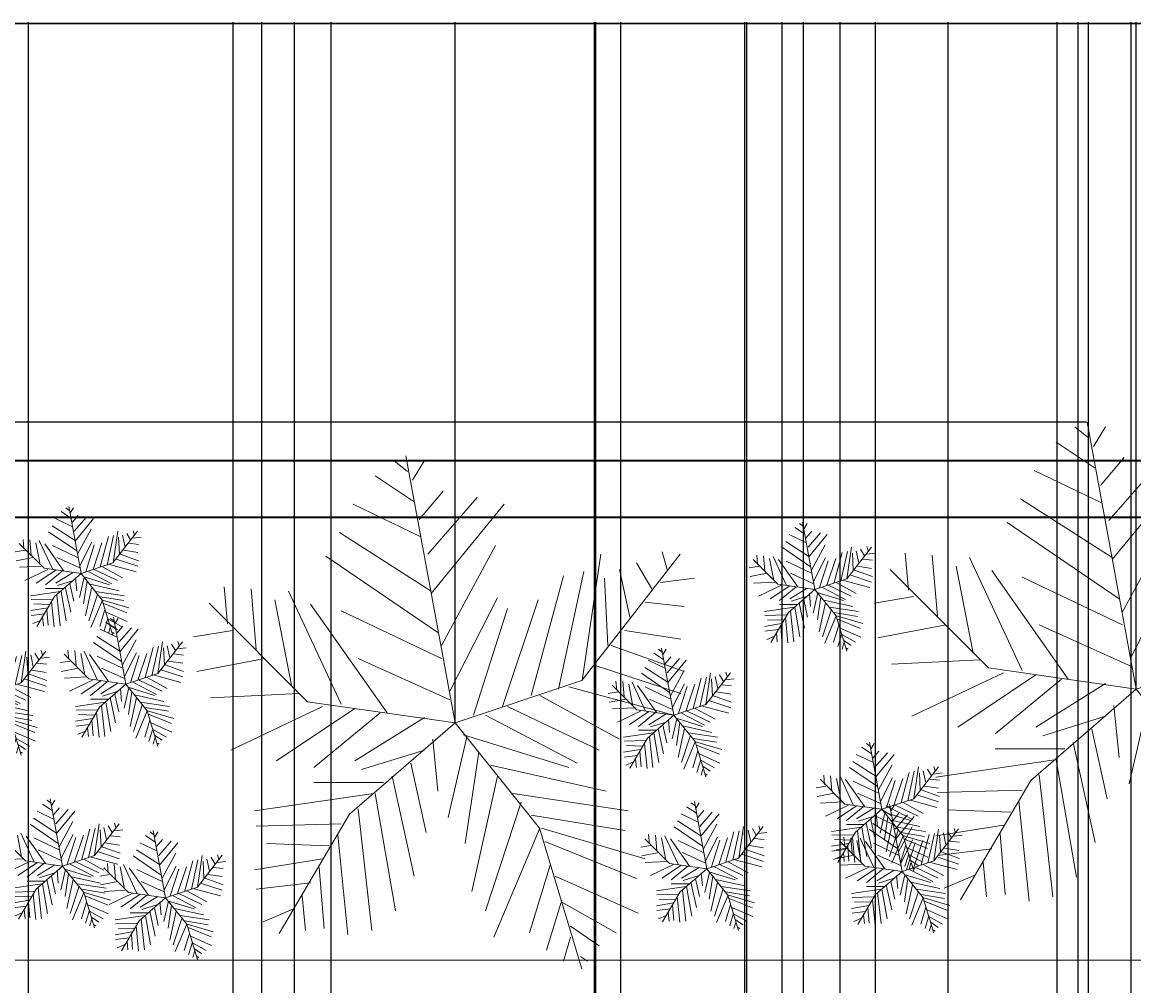
# Model space of a CAD drawing. Units: inches. Extents: x 818 to 1898, y 976 to 2364.
# Tile 79 of 96: x 1083 to 1259, y 2211 to 2364. Entities that reach past the tile are written whole.
import ezdxf

# ---------------------------------------------------------------- set-up
doc = ezdxf.new("R2010")
doc.units = ezdxf.units.IN
doc.header["$LTSCALE"] = 5
doc.header["$MEASUREMENT"] = 0
for name, color, linetype, lineweight in [('A-ANNO-DIMS', 2, 'Continuous', 18), ('C-PROP', 7, 'Continuous', 35), ('L-PLNT-BEDS', 94, 'Continuous', 18)]:
    doc.layers.add(name, color=color, linetype=linetype, lineweight=lineweight)
doc.layers.add('L-PLNT', color=116, linetype='Continuous', lineweight=13, true_color=0x136734)
doc.styles.get("Standard").update_dxf_attribs({"font": 'arial.ttf'})
doc.dimstyles.get("Standard").update_dxf_attribs({"dimtxt": 0.18, "dimasz": 0.18, "dimexe": 0.18, "dimexo": 0.0625, "dimgap": 0.09, "dimtad": 0, "dimtih": 1, "dimtoh": 1, "dimdec": 4, "dimzin": 0, "dimdsep": 46, "dimtxsty": 'Standard', "dimcen": 0.09, "dimadec": 0, "dimazin": 0, "dimtfac": 1, "dimtdec": 4, "dimtofl": 0, "dimtmove": 0, "dimatfit": 3, "dimfxl": 1, "dimtolj": 1, "dimtzin": 0, "dimarcsym": 0})

# ---------------------------------------------------------------- blocks, each defined once
blk = doc.blocks.new('SHRUB-ACCENT')
for p, q in [((8.8, 18.63), (7.25, 19.67)), ((8.53, 19.84), (7.99, 20.28)), ((10.44, 9.82), (8.47, 20.47)), ((8.74, 19.5), (9.21, 20.28)), ((9.08, 17.24), (6.37, 18.54)), ((9.01, 17.93), (9.96, 19.06)), ((9.35, 16.54), (11.31, 18.8)), ((9.48, 14.98), (12.39, 18.54)), ((9.75, 13.42), (5.28, 16.46)), ((9.48, 15.07), (5.82, 17.41)), ((9.89, 12.9), (12.06, 16.89)), ((15.49, 11.5), (19.41, 16.55)), ((15.51, 11.51), (16.25, 16.54)), ((17, 15.94), (17.41, 14.03)), ((17.68, 16.2), (18.29, 15.16)), ((18.69, 16.63), (18.9, 15.94)), ((4.55, 10.66), (0.62, 14.58)), ((1.35, 13.77), (1.22, 15.24)), ((2.3, 15.16), (2.51, 12.72)), ((3.25, 14.72), (3.93, 11.25)), ((3.79, 15.07), (5.89, 10.55)), ((7.72, 10.21), (4.67, 14.55)), ((5.89, 14.29), (9.89, 12.38)), ((10.23, 11.07), (12.12, 14.81)), ((11.17, 10.12), (12.53, 14.37)), ((12.33, 10.47), (13.75, 14.72)), ((13.48, 10.9), (14.76, 15.68)), ((14.56, 11.16), (15.58, 15.85)), ((16.39, 15.59), (16.53, 12.9)), ((18.02, 14.63), (19.57, 14.46)), ((18.62, 15.42), (19.98, 15.59)), ((1.56, 13.51), (0, 13.25)), ((2.84, 12.38), (0.14, 11.86)), ((6.57, 12.38), (10.23, 10.73)), ((16.66, 12.9), (19.57, 11.86)), ((17.2, 13.51), (19.44, 13.16)), ((4.2, 10.99), (0.68, 10.81)), ((10.44, 9.82), (4.55, 10.66)), ((10.44, 9.82), (15.49, 11.5)), ((13.82, 10.9), (17, 9.16)), ((14.97, 11.25), (19.17, 10.12)), ((15.98, 12.12), (19.44, 10.99)), ((5.15, 10.47), (1.49, 8.73)), ((6.43, 10.38), (3.32, 8.3)), ((7.45, 10.21), (4.81, 8.04)), ((10.44, 9.82), (6.23, 6.17)), ((9.21, 10.03), (6.43, 8.3)), ((9.55, 9.16), (9.75, 7.08)), ((10.9, 9.25), (10.16, 6.04)), ((10.44, 9.82), (13.8, 5.61)), ((10.77, 9.34), (14.97, 8.04)), ((11.65, 10.12), (15.31, 8.21)), ((12.53, 10.47), (16.19, 8.73)), ((7.59, 7.43), (4.81, 7.43)), ((9.21, 8.73), (6.7, 7.95)), ((7.92, 7.69), (8.8, 3.69)), ((8.67, 8.21), (9.28, 5.43)), ((11.38, 8.64), (10.84, 5)), ((12.12, 7.69), (11.11, 3.09)), ((11.85, 8.12), (16.46, 7.08)), ((7.18, 6.99), (2.44, 6.3)), ((5.89, 5.78), (2.51, 5.69)), ((6.23, 6.17), (3.43, 1.4)), ((5.76, 5.34), (6.16, 1.35)), ((6.57, 6.39), (7.11, 1.52)), ((7.25, 6.99), (8.06, 2.31)), ((13.07, 6.65), (11.65, 2.31)), ((13.82, 5.6), (11.99, 1.26)), ((12.73, 6.99), (17.34, 6.3)), ((13.48, 6.13), (17.2, 5.52)), ((13.8, 5.61), (15.49, 0)), ((13.88, 5.6), (18.02, 4.39)), ((5.15, 4.39), (2.44, 3.95)), ((5.42, 4.91), (2.91, 5)), ((5.01, 4.04), (5.21, 1.61)), ((14.22, 4.13), (13.41, 1.44)), ((14.02, 5.08), (17.68, 3.61)), ((14.43, 3.69), (17.74, 2.22)), ((4.67, 3.43), (2.51, 3.17)), ((4, 2.39), (2.78, 1.87)), ((4.33, 2.91), (4.47, 1.52)), ((14.7, 2.74), (14.09, 0.74)), ((14.7, 2.65), (16.86, 1.44)), ((15.04, 1.26), (14.76, 0.31)), ((15.04, 1.7), (16.19, 0.92)), ((15.44, 0.48), (15.71, 0.31))]:
    blk.add_line(p, q)
blk = doc.blocks.new('PALM-BORDER')
for p, q in [((41.53, 39.05), (33.72, 81.45)), ((33.95, 78.95), (31.8, 80.68)), ((34.76, 77.57), (36.65, 80.68)), ((35.03, 74.11), (28.83, 78.26)), ((35.84, 71.35), (39.61, 75.84)), ((37.18, 65.82), (45, 74.8)), ((36.11, 68.59), (25.33, 73.77)), ((37.72, 59.6), (49.31, 73.77)), ((37.72, 59.95), (23.17, 69.28)), ((39.34, 51.31), (47.96, 67.2)), ((38.8, 53.39), (21.02, 65.48)), ((61.61, 45.75), (77.23, 65.83)), ((61.71, 45.79), (64.67, 65.82)), ((74.37, 66.17), (75.18, 63.4)), ((70.33, 64.44), (72.75, 60.3)), ((53.62, 43.37), (58.74, 62.37)), ((57.93, 44.41), (61.97, 63.06)), ((65.21, 62.02), (65.75, 51.31)), ((67.63, 63.4), (69.25, 55.81)), ((74.1, 61.33), (79.49, 62.02)), ((5.39, 54.77), (4.85, 60.64)), ((9.16, 60.3), (9.97, 50.62)), ((12.93, 58.57), (15.63, 44.75)), ((15.09, 59.95), (23.44, 41.99)), ((40.69, 44.06), (48.23, 58.91)), ((49.04, 41.64), (54.7, 58.57)), ((71.68, 58.22), (77.87, 57.53)), ((18.1, 42.4), (2.48, 58.02)), ((30.72, 40.61), (18.59, 57.88)), ((23.44, 56.84), (39.34, 49.24)), ((44.46, 40.26), (49.85, 57.19)), ((6.2, 53.73), (0, 52.7)), ((68.44, 53.73), (77.33, 52.35)), ((66.29, 51.31), (77.87, 47.17)), ((11.32, 49.24), (0.54, 47.17)), ((26.14, 49.24), (40.69, 42.68)), ((63.59, 48.21), (77.33, 43.71)), ((41.53, 39.05), (61.61, 45.75)), ((59.55, 44.75), (76.26, 40.26)), ((16.71, 43.71), (2.69, 43.02)), ((41.53, 39.05), (18.1, 42.4)), ((54.97, 43.37), (67.63, 36.46)), ((20.48, 41.64), (5.93, 34.73)), ((25.6, 41.3), (13.2, 33.01)), ((29.64, 40.61), (19.13, 31.97)), ((49.85, 41.64), (64.4, 34.73)), ((41.53, 39.05), (24.79, 24.55)), ((36.65, 39.91), (25.6, 33.01)), ((41.53, 39.05), (54.92, 22.32)), ((46.35, 40.26), (60.9, 32.66)), ((42.84, 37.15), (59.55, 31.97)), ((37.99, 36.46), (38.8, 28.17)), ((43.38, 36.81), (40.42, 24.02)), ((36.65, 34.73), (26.68, 31.62)), ((45.27, 34.39), (43.11, 19.88)), ((34.49, 32.66), (36.92, 21.61)), ((47.15, 32.32), (65.48, 28.17)), ((31.53, 30.59), (35.03, 14.7)), ((48.23, 30.59), (44.19, 12.28)), ((30.18, 29.55), (19.13, 29.55)), ((28.56, 27.82), (9.7, 25.06)), ((28.83, 27.82), (32.07, 9.17)), ((50.66, 27.82), (68.98, 25.06)), ((26.14, 25.41), (28.29, 6.06)), ((52, 26.44), (46.35, 9.17)), ((23.44, 22.99), (9.97, 22.64)), ((24.79, 24.55), (13.63, 5.58)), ((53.62, 24.37), (68.44, 21.95)), ((22.9, 21.26), (24.52, 5.37)), ((54.97, 22.3), (47.69, 5.02)), ((54.92, 22.32), (61.61, 0)), ((55.24, 22.3), (71.68, 17.46)), ((21.56, 19.53), (11.59, 19.88)), ((55.78, 20.22), (70.33, 14.35)), ((20.48, 17.46), (9.7, 15.73)), ((19.94, 16.08), (20.75, 6.41)), ((56.59, 16.42), (53.35, 5.72)), ((57.39, 14.7), (70.6, 8.83)), ((18.59, 13.66), (9.97, 12.62)), ((17.24, 11.59), (17.78, 6.06)), ((58.47, 10.9), (56.05, 2.95)), ((15.9, 9.52), (11.05, 7.44)), ((58.47, 10.55), (67.09, 5.72)), ((59.82, 6.75), (64.4, 3.64)), ((59.82, 5.02), (58.74, 1.22)), ((61.44, 1.92), (62.51, 1.22))]:
    blk.add_line(p, q)
blk = doc.blocks.new('*D57')
at = {"layer": 'A-ANNO-DIMS', "color": 0, "lineweight": -2, "ltscale": 5, "transparency": 16777216}
for p, q in [((992.73, 2294.28), (992.73, 2363.87)), ((992.91, 2363.69), (1395.43, 2363.69)), ((1798.54, 2363.69), (1396.01, 2363.69)), ((1798.72, 2294.28), (1798.72, 2363.87))]:
    blk.add_line(p, q, dxfattribs=at)
at = {"layer": 'A-ANNO-DIMS', "color": 0, "ltscale": 5, "transparency": 16777216}
for points in [[(992.91, 2363.72), (992.91, 2363.66), (992.73, 2363.69)], [(1798.54, 2363.72), (1798.54, 2363.66), (1798.72, 2363.69)]]:
    blk.add_solid(points, dxfattribs=at)
at = {"layer": 'Defpoints', "color": 0, "ltscale": 5, "transparency": 16777216}
for p in [(1798.72, 2363.69), (992.73, 2294.22), (1798.72, 2294.22)]:
    blk.add_point(p, dxfattribs=at)
at = {"layer": 'A-ANNO-DIMS', "color": 0, "ltscale": 5, "transparency": 16777216, "insert": (1395.72, 2363.69), "char_height": 0.18, "attachment_point": 5}
blk.add_mtext('\\A1;806', dxfattribs=at)
blk = doc.blocks.new('*D59')
at = {"layer": 'A-ANNO-DIMS', "color": 0, "lineweight": -2, "ltscale": 5, "transparency": 16777216}
for p, q in [((1251.64, 2300.39), (818.03, 2300.39)), ((818.21, 2300.21), (818.21, 1669.95)), ((818.21, 1039.32), (818.21, 1669.59)), ((896.05, 1039.14), (818.03, 1039.14))]:
    blk.add_line(p, q, dxfattribs=at)
at = {"layer": 'A-ANNO-DIMS', "color": 0, "ltscale": 5, "transparency": 16777216}
for points in [[(818.18, 2300.21), (818.24, 2300.21), (818.21, 2300.39)], [(818.18, 1039.32), (818.24, 1039.32), (818.21, 1039.14)]]:
    blk.add_solid(points, dxfattribs=at)
at = {"layer": 'Defpoints', "color": 0, "ltscale": 5, "transparency": 16777216}
for p in [(818.21, 2300.39), (1251.71, 2300.39), (896.11, 1039.14)]:
    blk.add_point(p, dxfattribs=at)
at = {"layer": 'A-ANNO-DIMS', "color": 0, "ltscale": 5, "transparency": 16777216, "insert": (818.21, 1669.77), "char_height": 0.18, "attachment_point": 5}
blk.add_mtext('\\A1;1261.2', dxfattribs=at)
blk = doc.blocks.new('*D61')
at = {"layer": 'A-ANNO-DIMS', "color": 0, "lineweight": -2, "ltscale": 5, "transparency": 16777216}
for p, q in [((1071.73, 1203.03), (1071.73, 2363.87)), ((1071.91, 2363.69), (1250.94, 2363.69)), ((1430.55, 2363.69), (1251.51, 2363.69)), ((1430.73, 1203.03), (1430.73, 2363.87))]:
    blk.add_line(p, q, dxfattribs=at)
at = {"layer": 'A-ANNO-DIMS', "color": 0, "ltscale": 5, "transparency": 16777216}
for points in [[(1071.91, 2363.72), (1071.91, 2363.66), (1071.73, 2363.69)], [(1430.55, 2363.72), (1430.55, 2363.66), (1430.73, 2363.69)]]:
    blk.add_solid(points, dxfattribs=at)
at = {"layer": 'Defpoints', "color": 0, "ltscale": 5, "transparency": 16777216}
for p in [(1430.73, 2363.69), (1071.73, 1202.96), (1430.73, 1202.96)]:
    blk.add_point(p, dxfattribs=at)
at = {"layer": 'A-ANNO-DIMS', "color": 0, "ltscale": 5, "transparency": 16777216, "insert": (1251.23, 2363.69), "char_height": 0.18, "attachment_point": 5}
blk.add_mtext('\\A1;359', dxfattribs=at)
blk = doc.blocks.new('*D64')
at = {"layer": 'A-ANNO-DIMS', "color": 0, "lineweight": -2, "ltscale": 5, "transparency": 16777216}
for p, q in [((1197.73, 1501.14), (1197.73, 2363.87)), ((1197.91, 2363.69), (1313.93, 2363.69)), ((1430.55, 2363.69), (1314.52, 2363.69)), ((1430.73, 1501.14), (1430.73, 2363.87))]:
    blk.add_line(p, q, dxfattribs=at)
at = {"layer": 'A-ANNO-DIMS', "color": 0, "ltscale": 5, "transparency": 16777216}
for points in [[(1197.91, 2363.72), (1197.91, 2363.66), (1197.73, 2363.69)], [(1430.55, 2363.72), (1430.55, 2363.66), (1430.73, 2363.69)]]:
    blk.add_solid(points, dxfattribs=at)
at = {"layer": 'Defpoints', "color": 0, "ltscale": 5, "transparency": 16777216}
for p in [(1430.73, 2363.69), (1197.73, 1501.08), (1430.73, 1501.08)]:
    blk.add_point(p, dxfattribs=at)
at = {"layer": 'A-ANNO-DIMS', "color": 0, "ltscale": 5, "transparency": 16777216, "insert": (1314.23, 2363.69), "char_height": 0.18, "attachment_point": 5}
blk.add_mtext('\\A1;233', dxfattribs=at)
blk = doc.blocks.new('*D82')
at = {"layer": 'A-ANNO-DIMS', "color": 0, "lineweight": -2, "ltscale": 5, "transparency": 16777216}
for p, q in [((1083.73, 1501.14), (1083.73, 2363.87)), ((1083.91, 2363.69), (1140.45, 2363.69)), ((1197.55, 2363.69), (1141.01, 2363.69)), ((1197.73, 1501.14), (1197.73, 2363.87))]:
    blk.add_line(p, q, dxfattribs=at)
at = {"layer": 'A-ANNO-DIMS', "color": 0, "ltscale": 5, "transparency": 16777216}
for points in [[(1083.91, 2363.72), (1083.91, 2363.66), (1083.73, 2363.69)], [(1197.55, 2363.72), (1197.55, 2363.66), (1197.73, 2363.69)]]:
    blk.add_solid(points, dxfattribs=at)
at = {"layer": 'Defpoints', "color": 0, "ltscale": 5, "transparency": 16777216}
for p in [(1197.73, 2363.69), (1083.73, 1501.08), (1197.73, 1501.08)]:
    blk.add_point(p, dxfattribs=at)
at = {"layer": 'A-ANNO-DIMS', "color": 0, "ltscale": 5, "transparency": 16777216, "insert": (1140.73, 2363.69), "char_height": 0.18, "attachment_point": 5}
blk.add_mtext('\\A1;114', dxfattribs=at)
blk = doc.blocks.new('*D83')
at = {"layer": 'A-ANNO-DIMS', "color": 0, "lineweight": -2, "ltscale": 5, "transparency": 16777216}
for p, q in [((1197.73, 1700.14), (1197.73, 2363.87)), ((1197.91, 2363.69), (1228.02, 2363.69)), ((1258.55, 2363.69), (1228.43, 2363.69)), ((1258.73, 1700.14), (1258.73, 2363.87))]:
    blk.add_line(p, q, dxfattribs=at)
at = {"layer": 'A-ANNO-DIMS', "color": 0, "ltscale": 5, "transparency": 16777216}
for points in [[(1197.91, 2363.72), (1197.91, 2363.66), (1197.73, 2363.69)], [(1258.55, 2363.72), (1258.55, 2363.66), (1258.73, 2363.69)]]:
    blk.add_solid(points, dxfattribs=at)
at = {"layer": 'Defpoints', "color": 0, "ltscale": 5, "transparency": 16777216}
for p in [(1258.73, 2363.69), (1197.73, 1700.08), (1258.73, 1700.08)]:
    blk.add_point(p, dxfattribs=at)
at = {"layer": 'A-ANNO-DIMS', "color": 0, "ltscale": 5, "transparency": 16777216, "insert": (1228.23, 2363.69), "char_height": 0.18, "attachment_point": 5}
blk.add_mtext('\\A1;61', dxfattribs=at)
blk = doc.blocks.new('*D86')
at = {"layer": 'A-ANNO-DIMS', "color": 0, "lineweight": -2, "ltscale": 5, "transparency": 16777216}
for p, q in [((1258.73, 2053.14), (1258.73, 2363.87)), ((1258.91, 2363.69), (1486.43, 2363.69)), ((1714.55, 2363.69), (1487.02, 2363.69)), ((1714.73, 2053.14), (1714.73, 2363.87))]:
    blk.add_line(p, q, dxfattribs=at)
at = {"layer": 'A-ANNO-DIMS', "color": 0, "ltscale": 5, "transparency": 16777216}
for points in [[(1258.91, 2363.72), (1258.91, 2363.66), (1258.73, 2363.69)], [(1714.55, 2363.72), (1714.55, 2363.66), (1714.73, 2363.69)]]:
    blk.add_solid(points, dxfattribs=at)
at = {"layer": 'Defpoints', "color": 0, "ltscale": 5, "transparency": 16777216}
for p in [(1714.73, 2363.69), (1258.73, 2053.08), (1714.73, 2053.08)]:
    blk.add_point(p, dxfattribs=at)
at = {"layer": 'A-ANNO-DIMS', "color": 0, "ltscale": 5, "transparency": 16777216, "insert": (1486.73, 2363.69), "char_height": 0.18, "attachment_point": 5}
blk.add_mtext('\\A1;456', dxfattribs=at)
blk = doc.blocks.new('*D87')
at = {"layer": 'A-ANNO-DIMS', "color": 0, "lineweight": -2, "ltscale": 5, "transparency": 16777216}
for p, q in [((992.73, 2294.28), (992.73, 2363.87)), ((992.91, 2363.69), (1038.02, 2363.69)), ((1083.55, 2363.69), (1038.43, 2363.69)), ((1083.73, 2206.03), (1083.73, 2363.87))]:
    blk.add_line(p, q, dxfattribs=at)
at = {"layer": 'A-ANNO-DIMS', "color": 0, "ltscale": 5, "transparency": 16777216}
for points in [[(992.91, 2363.72), (992.91, 2363.66), (992.73, 2363.69)], [(1083.55, 2363.72), (1083.55, 2363.66), (1083.73, 2363.69)]]:
    blk.add_solid(points, dxfattribs=at)
at = {"layer": 'Defpoints', "color": 0, "ltscale": 5, "transparency": 16777216}
for p in [(1083.73, 2363.69), (992.73, 2294.22), (1083.73, 2205.97)]:
    blk.add_point(p, dxfattribs=at)
at = {"layer": 'A-ANNO-DIMS', "color": 0, "ltscale": 5, "transparency": 16777216, "insert": (1038.23, 2363.69), "char_height": 0.18, "attachment_point": 5}
blk.add_mtext('\\A1;91', dxfattribs=at)
blk = doc.blocks.new('*D93')
at = {"layer": 'A-ANNO-DIMS', "color": 0, "lineweight": -2, "ltscale": 5, "transparency": 16777216}
for p, q in [((1068.34, 1071.12), (1068.34, 2363.87)), ((1068.52, 2363.69), (1094.16, 2363.69)), ((1120.58, 2363.69), (1094.94, 2363.69)), ((1120.76, 1071.12), (1120.76, 2363.87))]:
    blk.add_line(p, q, dxfattribs=at)
at = {"layer": 'A-ANNO-DIMS', "color": 0, "ltscale": 5, "transparency": 16777216}
for points in [[(1068.52, 2363.72), (1068.52, 2363.66), (1068.34, 2363.69)], [(1120.58, 2363.72), (1120.58, 2363.66), (1120.76, 2363.69)]]:
    blk.add_solid(points, dxfattribs=at)
at = {"layer": 'Defpoints', "color": 0, "ltscale": 5, "transparency": 16777216}
for p in [(1120.76, 2363.69), (1068.34, 1071.06), (1120.76, 1071.06)]:
    blk.add_point(p, dxfattribs=at)
at = {"layer": 'A-ANNO-DIMS', "color": 0, "ltscale": 5, "transparency": 16777216, "insert": (1094.55, 2363.69), "char_height": 0.18, "attachment_point": 5}
blk.add_mtext('\\A1;52.42', dxfattribs=at)
blk = doc.blocks.new('*D94')
at = {"layer": 'A-ANNO-DIMS', "color": 0, "lineweight": -2, "ltscale": 5, "transparency": 16777216}
for p, q in [((1120.76, 1071.12), (1120.76, 2363.87)), ((1120.94, 2363.69), (1146.76, 2363.69)), ((1173.36, 2363.69), (1147.55, 2363.69)), ((1173.54, 1071.12), (1173.54, 2363.87))]:
    blk.add_line(p, q, dxfattribs=at)
at = {"layer": 'A-ANNO-DIMS', "color": 0, "ltscale": 5, "transparency": 16777216}
for points in [[(1120.94, 2363.72), (1120.94, 2363.66), (1120.76, 2363.69)], [(1173.36, 2363.72), (1173.36, 2363.66), (1173.54, 2363.69)]]:
    blk.add_solid(points, dxfattribs=at)
at = {"layer": 'Defpoints', "color": 0, "ltscale": 5, "transparency": 16777216}
for p in [(1173.54, 2363.69), (1120.76, 1071.06), (1173.54, 1071.06)]:
    blk.add_point(p, dxfattribs=at)
at = {"layer": 'A-ANNO-DIMS', "color": 0, "ltscale": 5, "transparency": 16777216, "insert": (1147.15, 2363.69), "char_height": 0.18, "attachment_point": 5}
blk.add_mtext('\\A1;52.78', dxfattribs=at)
blk = doc.blocks.new('*D95')
at = {"layer": 'A-ANNO-DIMS', "color": 0, "lineweight": -2, "ltscale": 5, "transparency": 16777216}
for p, q in [((1173.54, 1071.12), (1173.54, 2363.87)), ((1173.72, 2363.69), (1201.29, 2363.69)), ((1229.47, 2363.69), (1201.9, 2363.69)), ((1229.65, 1071.12), (1229.65, 2363.87))]:
    blk.add_line(p, q, dxfattribs=at)
at = {"layer": 'A-ANNO-DIMS', "color": 0, "ltscale": 5, "transparency": 16777216}
for points in [[(1173.72, 2363.72), (1173.72, 2363.66), (1173.54, 2363.69)], [(1229.47, 2363.72), (1229.47, 2363.66), (1229.65, 2363.69)]]:
    blk.add_solid(points, dxfattribs=at)
at = {"layer": 'Defpoints', "color": 0, "ltscale": 5, "transparency": 16777216}
for p in [(1229.65, 2363.69), (1173.54, 1071.06), (1229.65, 1071.06)]:
    blk.add_point(p, dxfattribs=at)
at = {"layer": 'A-ANNO-DIMS', "color": 0, "ltscale": 5, "transparency": 16777216, "insert": (1201.59, 2363.69), "char_height": 0.18, "attachment_point": 5}
blk.add_mtext('\\A1;56.1', dxfattribs=at)
blk = doc.blocks.new('*D96')
at = {"layer": 'A-ANNO-DIMS', "color": 0, "lineweight": -2, "ltscale": 5, "transparency": 16777216}
for p, q in [((1229.65, 1071.12), (1229.65, 2363.87)), ((1229.83, 2363.69), (1256.52, 2363.69)), ((1283.99, 2363.69), (1257.3, 2363.69)), ((1284.17, 1071.12), (1284.17, 2363.87))]:
    blk.add_line(p, q, dxfattribs=at)
at = {"layer": 'A-ANNO-DIMS', "color": 0, "ltscale": 5, "transparency": 16777216}
for points in [[(1229.83, 2363.72), (1229.83, 2363.66), (1229.65, 2363.69)], [(1283.99, 2363.72), (1283.99, 2363.66), (1284.17, 2363.69)]]:
    blk.add_solid(points, dxfattribs=at)
at = {"layer": 'Defpoints', "color": 0, "ltscale": 5, "transparency": 16777216}
for p in [(1284.17, 2363.69), (1229.65, 1071.06), (1284.17, 1071.06)]:
    blk.add_point(p, dxfattribs=at)
at = {"layer": 'A-ANNO-DIMS', "color": 0, "ltscale": 5, "transparency": 16777216, "insert": (1256.91, 2363.69), "char_height": 0.18, "attachment_point": 5}
blk.add_mtext('\\A1;54.52', dxfattribs=at)
blk = doc.blocks.new('*D109')
at = {"layer": 'A-ANNO-DIMS', "color": 0, "lineweight": -2, "ltscale": 5, "transparency": 16777216}
for p, q in [((1125.92, 1410.12), (1125.92, 2363.87)), ((1126.1, 2363.69), (1164.25, 2363.69)), ((1203.15, 2363.69), (1165, 2363.69)), ((1203.33, 1409.91), (1203.33, 2363.87))]:
    blk.add_line(p, q, dxfattribs=at)
at = {"layer": 'A-ANNO-DIMS', "color": 0, "ltscale": 5, "transparency": 16777216}
for points in [[(1126.1, 2363.72), (1126.1, 2363.66), (1125.92, 2363.69)], [(1203.15, 2363.72), (1203.15, 2363.66), (1203.33, 2363.69)]]:
    blk.add_solid(points, dxfattribs=at)
at = {"layer": 'Defpoints', "color": 0, "ltscale": 5, "transparency": 16777216}
for p in [(1203.33, 2363.69), (1125.92, 1410.05), (1203.33, 1409.85)]:
    blk.add_point(p, dxfattribs=at)
at = {"layer": 'A-ANNO-DIMS', "color": 0, "ltscale": 5, "transparency": 16777216, "insert": (1164.62, 2363.69), "char_height": 0.18, "attachment_point": 5}
blk.add_mtext('\\A1;77.41', dxfattribs=at)
blk = doc.blocks.new('*D123')
at = {"layer": 'A-ANNO-DIMS', "color": 0, "lineweight": -2, "ltscale": 5, "transparency": 16777216}
for p, q in [((1083.73, 2044.14), (1083.73, 2363.87)), ((1083.91, 2363.69), (1107.35, 2363.69)), ((1131.59, 2363.69), (1108.14, 2363.69)), ((1131.77, 1974.64), (1131.77, 2363.87))]:
    blk.add_line(p, q, dxfattribs=at)
at = {"layer": 'A-ANNO-DIMS', "color": 0, "ltscale": 5, "transparency": 16777216}
for points in [[(1083.91, 2363.72), (1083.91, 2363.66), (1083.73, 2363.69)], [(1131.59, 2363.72), (1131.59, 2363.66), (1131.77, 2363.69)]]:
    blk.add_solid(points, dxfattribs=at)
at = {"layer": 'Defpoints', "color": 0, "ltscale": 5, "transparency": 16777216}
for p in [(1131.77, 2363.69), (1083.73, 2044.08), (1131.77, 1974.57)]:
    blk.add_point(p, dxfattribs=at)
at = {"layer": 'A-ANNO-DIMS', "color": 0, "ltscale": 5, "transparency": 16777216, "insert": (1107.75, 2363.69), "char_height": 0.18, "attachment_point": 5}
blk.add_mtext('\\A1;48.04', dxfattribs=at)
blk = doc.blocks.new('*D126')
at = {"layer": 'A-ANNO-DIMS', "color": 0, "lineweight": -2, "ltscale": 5, "transparency": 16777216}
for p, q in [((1035.38, 1252.09), (1035.38, 2363.87)), ((1035.56, 2363.69), (1075.41, 2363.69)), ((1116.01, 2363.69), (1076.16, 2363.69)), ((1116.19, 1236.03), (1116.19, 2363.87))]:
    blk.add_line(p, q, dxfattribs=at)
at = {"layer": 'A-ANNO-DIMS', "color": 0, "ltscale": 5, "transparency": 16777216}
for points in [[(1035.56, 2363.72), (1035.56, 2363.66), (1035.38, 2363.69)], [(1116.01, 2363.72), (1116.01, 2363.66), (1116.19, 2363.69)]]:
    blk.add_solid(points, dxfattribs=at)
at = {"layer": 'Defpoints', "color": 0, "ltscale": 5, "transparency": 16777216}
for p in [(1035.38, 2363.69), (1035.38, 1252.02), (1116.19, 1235.96)]:
    blk.add_point(p, dxfattribs=at)
at = {"layer": 'A-ANNO-DIMS', "color": 0, "ltscale": 5, "transparency": 16777216, "insert": (1075.78, 2363.69), "char_height": 0.18, "attachment_point": 5}
blk.add_mtext('\\A1;80.81', dxfattribs=at)
blk = doc.blocks.new('*D135')
at = {"layer": 'A-ANNO-DIMS', "color": 0, "lineweight": -2, "ltscale": 5, "transparency": 16777216}
for p, q in [((1041.7, 2252.7), (1041.7, 2363.87)), ((1041.88, 2363.69), (1096.11, 2363.69)), ((1151.25, 2363.69), (1097.02, 2363.69)), ((1151.43, 2252.7), (1151.43, 2363.87))]:
    blk.add_line(p, q, dxfattribs=at)
at = {"layer": 'A-ANNO-DIMS', "color": 0, "ltscale": 5, "transparency": 16777216}
for points in [[(1041.88, 2363.72), (1041.88, 2363.66), (1041.7, 2363.69)], [(1151.25, 2363.72), (1151.25, 2363.66), (1151.43, 2363.69)]]:
    blk.add_solid(points, dxfattribs=at)
at = {"layer": 'Defpoints', "color": 0, "ltscale": 5, "transparency": 16777216}
for p in [(1151.43, 2363.69), (1041.7, 2252.64), (1151.43, 2252.64)]:
    blk.add_point(p, dxfattribs=at)
at = {"layer": 'A-ANNO-DIMS', "color": 0, "ltscale": 5, "transparency": 16777216, "insert": (1096.56, 2363.69), "char_height": 0.18, "attachment_point": 5}
blk.add_mtext('\\A1;109.72', dxfattribs=at)
blk = doc.blocks.new('*D136')
at = {"layer": 'A-ANNO-DIMS', "color": 0, "lineweight": -2, "ltscale": 5, "transparency": 16777216}
for p, q in [((1151.43, 2252.7), (1151.43, 2363.87)), ((1151.61, 2363.69), (1205.1, 2363.69)), ((1259.34, 2363.69), (1205.84, 2363.69)), ((1259.52, 2258.06), (1259.52, 2363.87))]:
    blk.add_line(p, q, dxfattribs=at)
at = {"layer": 'A-ANNO-DIMS', "color": 0, "ltscale": 5, "transparency": 16777216}
for points in [[(1151.61, 2363.72), (1151.61, 2363.66), (1151.43, 2363.69)], [(1259.34, 2363.72), (1259.34, 2363.66), (1259.52, 2363.69)]]:
    blk.add_solid(points, dxfattribs=at)
at = {"layer": 'Defpoints', "color": 0, "ltscale": 5, "transparency": 16777216}
for p in [(1259.52, 2363.69), (1259.52, 2257.99), (1151.43, 2252.64)]:
    blk.add_point(p, dxfattribs=at)
at = {"layer": 'A-ANNO-DIMS', "color": 0, "ltscale": 5, "transparency": 16777216, "insert": (1205.47, 2363.69), "char_height": 0.18, "attachment_point": 5}
blk.add_mtext('\\A1;108.1', dxfattribs=at)
blk = doc.blocks.new('*D140')
at = {"layer": 'A-ANNO-DIMS', "color": 0, "lineweight": -2, "ltscale": 5, "transparency": 16777216}
for p, q in [((1083.73, 2053.14), (1083.73, 2363.87)), ((1083.91, 2363.69), (1150.46, 2363.69)), ((1217.93, 2363.69), (1151.37, 2363.69)), ((1218.11, 2083.32), (1218.11, 2363.87))]:
    blk.add_line(p, q, dxfattribs=at)
at = {"layer": 'A-ANNO-DIMS', "color": 0, "ltscale": 5, "transparency": 16777216}
for points in [[(1083.91, 2363.72), (1083.91, 2363.66), (1083.73, 2363.69)], [(1217.93, 2363.72), (1217.93, 2363.66), (1218.11, 2363.69)]]:
    blk.add_solid(points, dxfattribs=at)
at = {"layer": 'Defpoints', "color": 0, "ltscale": 5, "transparency": 16777216}
for p in [(1218.11, 2363.69), (1218.11, 2083.26), (1083.73, 2053.08)]:
    blk.add_point(p, dxfattribs=at)
at = {"layer": 'A-ANNO-DIMS', "color": 0, "ltscale": 5, "transparency": 16777216, "insert": (1150.92, 2363.69), "char_height": 0.18, "attachment_point": 5}
blk.add_mtext('\\A1;134.39', dxfattribs=at)
blk = doc.blocks.new('*D143')
at = {"layer": 'A-ANNO-DIMS', "color": 0, "lineweight": -2, "ltscale": 5, "transparency": 16777216}
for p, q in [((1083.73, 2206.03), (1083.73, 2363.87)), ((1083.91, 2363.69), (1140.1, 2363.69)), ((1197.21, 2363.69), (1141.01, 2363.69)), ((1197.39, 2122.44), (1197.39, 2363.87))]:
    blk.add_line(p, q, dxfattribs=at)
at = {"layer": 'A-ANNO-DIMS', "color": 0, "ltscale": 5, "transparency": 16777216}
for points in [[(1083.91, 2363.72), (1083.91, 2363.66), (1083.73, 2363.69)], [(1197.21, 2363.72), (1197.21, 2363.66), (1197.39, 2363.69)]]:
    blk.add_solid(points, dxfattribs=at)
at = {"layer": 'Defpoints', "color": 0, "ltscale": 5, "transparency": 16777216}
for p in [(1197.39, 2363.69), (1083.73, 2205.97), (1197.39, 2122.38)]:
    blk.add_point(p, dxfattribs=at)
at = {"layer": 'A-ANNO-DIMS', "color": 0, "ltscale": 5, "transparency": 16777216, "insert": (1140.56, 2363.69), "char_height": 0.18, "attachment_point": 5}
blk.add_mtext('\\A1;113.67', dxfattribs=at)
blk = doc.blocks.new('*D144')
at = {"layer": 'A-ANNO-DIMS', "color": 0, "lineweight": -2, "ltscale": 5, "transparency": 16777216}
for p, q in [((1197.39, 2122.44), (1197.39, 2363.87)), ((1197.57, 2363.69), (1204.5, 2363.69)), ((1212.34, 2363.69), (1205.41, 2363.69)), ((1212.52, 2145.31), (1212.52, 2363.87))]:
    blk.add_line(p, q, dxfattribs=at)
at = {"layer": 'A-ANNO-DIMS', "color": 0, "ltscale": 5, "transparency": 16777216}
for points in [[(1197.57, 2363.72), (1197.57, 2363.66), (1197.39, 2363.69)], [(1212.34, 2363.72), (1212.34, 2363.66), (1212.52, 2363.69)]]:
    blk.add_solid(points, dxfattribs=at)
at = {"layer": 'Defpoints', "color": 0, "ltscale": 5, "transparency": 16777216}
for p in [(1212.52, 2363.69), (1212.52, 2145.25), (1197.39, 2122.38)]:
    blk.add_point(p, dxfattribs=at)
at = {"layer": 'A-ANNO-DIMS', "color": 0, "ltscale": 5, "transparency": 16777216, "insert": (1204.96, 2363.69), "char_height": 0.18, "attachment_point": 5}
blk.add_mtext('\\A1;15.128', dxfattribs=at)
blk = doc.blocks.new('*D158')
at = {"layer": 'A-ANNO-DIMS', "color": 0, "lineweight": -2, "ltscale": 5, "transparency": 16777216}
for p, q in [((1173.73, 1590.82), (1173.73, 2363.87)), ((1173.91, 2363.69), (1175.57, 2363.69)), ((1177.55, 2363.69), (1175.88, 2363.69)), ((1177.73, 1586.82), (1177.73, 2363.87))]:
    blk.add_line(p, q, dxfattribs=at)
at = {"layer": 'A-ANNO-DIMS', "color": 0, "ltscale": 5, "transparency": 16777216}
for points in [[(1173.91, 2363.72), (1173.91, 2363.66), (1173.73, 2363.69)], [(1177.55, 2363.72), (1177.55, 2363.66), (1177.73, 2363.69)]]:
    blk.add_solid(points, dxfattribs=at)
at = {"layer": 'Defpoints', "color": 0, "ltscale": 5, "transparency": 16777216}
for p in [(1177.73, 2363.69), (1173.73, 1590.76), (1177.73, 1586.76)]:
    blk.add_point(p, dxfattribs=at)
at = {"layer": 'A-ANNO-DIMS', "color": 0, "ltscale": 5, "transparency": 16777216, "insert": (1175.73, 2363.69), "char_height": 0.18, "attachment_point": 5}
blk.add_mtext('\\A1;4', dxfattribs=at)
blk = doc.blocks.new('*D269')
at = {"layer": 'A-ANNO-DIMS', "color": 0, "lineweight": -2, "ltscale": 5, "transparency": 16777216}
for p, q in [((1246.94, 1534.14), (1246.94, 2363.87)), ((1247.12, 2363.69), (1293.71, 2363.69)), ((1341.08, 2363.69), (1294.49, 2363.69)), ((1341.26, 1534.14), (1341.26, 2363.87))]:
    blk.add_line(p, q, dxfattribs=at)
at = {"layer": 'A-ANNO-DIMS', "color": 0, "ltscale": 5, "transparency": 16777216}
for points in [[(1247.12, 2363.72), (1247.12, 2363.66), (1246.94, 2363.69)], [(1341.08, 2363.72), (1341.08, 2363.66), (1341.26, 2363.69)]]:
    blk.add_solid(points, dxfattribs=at)
at = {"layer": 'Defpoints', "color": 0, "ltscale": 5, "transparency": 16777216}
for p in [(1341.26, 2363.69), (1246.94, 1534.08), (1341.26, 1534.08)]:
    blk.add_point(p, dxfattribs=at)
at = {"layer": 'A-ANNO-DIMS', "color": 0, "ltscale": 5, "transparency": 16777216, "insert": (1294.1, 2363.69), "char_height": 0.18, "attachment_point": 5}
blk.add_mtext('\\A1;94.32', dxfattribs=at)
blk = doc.blocks.new('*D271')
at = {"layer": 'A-ANNO-DIMS', "color": 0, "lineweight": -2, "ltscale": 5, "transparency": 16777216}
for p, q in [((1206.73, 1510.14), (1206.73, 2363.87)), ((1206.91, 2363.69), (1226.45, 2363.69)), ((1246.76, 2363.69), (1227.21, 2363.69)), ((1246.94, 1510.14), (1246.94, 2363.87))]:
    blk.add_line(p, q, dxfattribs=at)
at = {"layer": 'A-ANNO-DIMS', "color": 0, "ltscale": 5, "transparency": 16777216}
for points in [[(1206.91, 2363.72), (1206.91, 2363.66), (1206.73, 2363.69)], [(1246.76, 2363.72), (1246.76, 2363.66), (1246.94, 2363.69)]]:
    blk.add_solid(points, dxfattribs=at)
at = {"layer": 'Defpoints', "color": 0, "ltscale": 5, "transparency": 16777216}
for p in [(1246.94, 2363.69), (1206.73, 1510.08), (1246.94, 1510.08)]:
    blk.add_point(p, dxfattribs=at)
at = {"layer": 'A-ANNO-DIMS', "color": 0, "ltscale": 5, "transparency": 16777216, "insert": (1226.83, 2363.69), "char_height": 0.18, "attachment_point": 5}
blk.add_mtext('\\A1;40.21', dxfattribs=at)
blk = doc.blocks.new('*D276')
at = {"layer": 'A-ANNO-DIMS', "color": 0, "lineweight": -2, "ltscale": 5, "transparency": 16777216}
for p, q in [((1206.73, 1687.14), (1206.73, 2363.87)), ((1206.91, 2363.69), (1228.95, 2363.69)), ((1251.75, 2363.69), (1229.71, 2363.69)), ((1251.93, 1681.44), (1251.93, 2363.87))]:
    blk.add_line(p, q, dxfattribs=at)
at = {"layer": 'A-ANNO-DIMS', "color": 0, "ltscale": 5, "transparency": 16777216}
for points in [[(1206.91, 2363.72), (1206.91, 2363.66), (1206.73, 2363.69)], [(1251.75, 2363.72), (1251.75, 2363.66), (1251.93, 2363.69)]]:
    blk.add_solid(points, dxfattribs=at)
at = {"layer": 'Defpoints', "color": 0, "ltscale": 5, "transparency": 16777216}
for p in [(1251.93, 2363.69), (1206.73, 1687.08), (1251.93, 1681.38)]:
    blk.add_point(p, dxfattribs=at)
at = {"layer": 'A-ANNO-DIMS', "color": 0, "ltscale": 5, "transparency": 16777216, "insert": (1229.33, 2363.69), "char_height": 0.18, "attachment_point": 5}
blk.add_mtext('\\A1;45.21', dxfattribs=at)
blk = doc.blocks.new('*D281')
at = {"layer": 'A-ANNO-DIMS', "color": 0, "lineweight": -2, "ltscale": 5, "transparency": 16777216}
for p, q in [((1250.3, 1913.7), (1250.3, 2363.87)), ((1250.48, 2363.69), (1420.12, 2363.69)), ((1590.55, 2363.69), (1420.91, 2363.69)), ((1590.73, 2011.14), (1590.73, 2363.87))]:
    blk.add_line(p, q, dxfattribs=at)
at = {"layer": 'A-ANNO-DIMS', "color": 0, "ltscale": 5, "transparency": 16777216}
for points in [[(1250.48, 2363.72), (1250.48, 2363.66), (1250.3, 2363.69)], [(1590.55, 2363.72), (1590.55, 2363.66), (1590.73, 2363.69)]]:
    blk.add_solid(points, dxfattribs=at)
at = {"layer": 'Defpoints', "color": 0, "ltscale": 5, "transparency": 16777216}
for p in [(1590.73, 2363.69), (1590.73, 2011.08), (1250.3, 1913.64)]:
    blk.add_point(p, dxfattribs=at)
at = {"layer": 'A-ANNO-DIMS', "color": 0, "ltscale": 5, "transparency": 16777216, "insert": (1420.51, 2363.69), "char_height": 0.18, "attachment_point": 5}
blk.add_mtext('\\A1;340.4', dxfattribs=at)

msp = doc.modelspace()

# ---------------------------------------------------------------- linework, layer by layer
at = {"layer": 'C-PROP', "ltscale": 5}
for p, q in [((1798.7173, 2294.2171), (992.7251, 2294.2171)), ((1789.7173, 2285.2171), (1001.7252, 2285.2171))]:
    msp.add_line(p, q, dxfattribs=at)
at = {"layer": 'L-PLNT-BEDS', "ltscale": 5}
msp.add_line((1789.7173, 2214.9709), (1071.7251, 2214.9709), dxfattribs=at)

# ---------------------------------------------------------------- block references
at = {"layer": 'L-PLNT'}
for name, p in [('PALM-BORDER', (1217.9881, 2218.9437)), ('PALM-BORDER', (1109.8973, 2213.5896)), ('SHRUB-ACCENT', (1081.633, 2266.5141)), ('SHRUB-ACCENT', (1198.0857, 2263.9991)), ('SHRUB-ACCENT', (1088.7517, 2248.941)), ('SHRUB-ACCENT', (1067.0685, 2247.4883)), ('SHRUB-ACCENT', (1175.715, 2244.034)), ('SHRUB-ACCENT', (1208.7132, 2229.0843)), ('SHRUB-ACCENT', (1078.7017, 2220.0709)), ('SHRUB-ACCENT', (1180.917, 2219.648)), ('SHRUB-ACCENT', (1211.9044, 2219.2296)), ('SHRUB-ACCENT', (1095.0329, 2215.05))]:
    msp.add_blockref(name, p, dxfattribs=at)

# ---------------------------------------------------------------- dimensions: what is measured, and where the dimension line sits
at = {"layer": 'A-ANNO-DIMS', "ltscale": 5}
for base, p1, p2, override, picture, middle in [((1798.7173, 2363.6929), (992.7251, 2294.2171), (1798.7173, 2294.2171), {"dimdec": 0, "dimlfac": 1, "dimrnd": 0, "dimzin": 0, "dimdsep": 46, "dimlunit": 2}, '*D57', (1395.7212, 2363.6929)), ((1083.7251, 2363.6929), (992.7251, 2294.2171), (1083.7251, 2205.9709), {"dimdec": 0, "dimlfac": 1, "dimrnd": 0, "dimzin": 0, "dimdsep": 46, "dimlunit": 2}, '*D87', (1038.2251, 2363.6929)), ((1035.3768, 2363.6929), (1116.1882, 1235.9642), (1035.3768, 1252.0242), {"dimdec": 2, "dimlfac": 1, "dimrnd": 0, "dimzin": 0, "dimdsep": 46, "dimlunit": 2}, '*D126', (1075.7825, 2363.6929)), ((1151.4251, 2363.6929), (1041.7008, 2252.6408), (1151.4251, 2252.6408), {"dimdec": 2, "dimlfac": 1, "dimrnd": 0, "dimzin": 0, "dimdsep": 46, "dimlunit": 2}, '*D135', (1096.5629, 2363.6929)), ((1120.7618, 2363.6929), (1068.3377, 1071.0552), (1120.7618, 1071.0552), {"dimdec": 2, "dimlfac": 1, "dimrnd": 0, "dimzin": 0, "dimdsep": 46, "dimlunit": 2}, '*D93', (1094.5497, 2363.6929)), ((1430.7251, 2363.6929), (1071.7251, 1202.9642), (1430.7251, 1202.9642), {"dimdec": 0, "dimlfac": 1, "dimrnd": 0, "dimzin": 0, "dimdsep": 46, "dimlunit": 2}, '*D61', (1251.2251, 2363.6929)), ((1197.7251, 2363.6929), (1083.7251, 1501.0782), (1197.7251, 1501.0782), {"dimdec": 0, "dimlfac": 1, "dimrnd": 0, "dimzin": 0, "dimdsep": 46, "dimlunit": 2}, '*D82', (1140.7251, 2363.6929)), ((1131.7651, 2363.6929), (1083.7251, 2044.0782), (1131.7651, 1974.5735), {"dimdec": 2, "dimlfac": 1, "dimrnd": 0, "dimzin": 0, "dimdsep": 46, "dimlunit": 2}, '*D123', (1107.7451, 2363.6929)), ((1218.1114, 2363.6929), (1083.7251, 2053.0782), (1218.1114, 2083.2623), {"dimdec": 2, "dimlfac": 1, "dimrnd": 0, "dimzin": 0, "dimdsep": 46, "dimlunit": 2}, '*D140', (1150.9183, 2363.6929)), ((1197.3925, 2363.6929), (1083.7251, 2205.9709), (1197.3925, 2122.3767), {"dimdec": 2, "dimlfac": 1, "dimrnd": 0, "dimzin": 0, "dimdsep": 46, "dimlunit": 2}, '*D143', (1140.5588, 2363.6929)), ((1173.5418, 2363.6929), (1120.7618, 1071.0552), (1173.5418, 1071.0552), {"dimdec": 2, "dimlfac": 1, "dimrnd": 0, "dimzin": 0, "dimdsep": 46, "dimlunit": 2}, '*D94', (1147.1518, 2363.6929)), ((1203.3292, 2363.6929), (1125.9172, 1410.0547), (1203.3292, 1409.8484), {"dimdec": 2, "dimlfac": 1, "dimrnd": 0, "dimzin": 0, "dimdsep": 46, "dimlunit": 2}, '*D109', (1164.6232, 2363.6929)), ((1259.5159, 2363.6929), (1151.4251, 2252.6408), (1259.5159, 2257.9948), {"dimdec": 1, "dimlfac": 1, "dimrnd": 0, "dimzin": 0, "dimdsep": 46, "dimlunit": 2}, '*D136', (1205.4705, 2363.6929)), ((1229.6474, 2363.6929), (1173.5418, 1071.0552), (1229.6474, 1071.0552), {"dimdec": 1, "dimlfac": 1, "dimrnd": 0, "dimzin": 0, "dimdsep": 46, "dimlunit": 2}, '*D95', (1201.5946, 2363.6929)), ((1177.7251, 2363.6929), (1173.7251, 1590.7585), (1177.7251, 1586.7585), {"dimdec": 0, "dimlfac": 1, "dimrnd": 0, "dimzin": 0, "dimdsep": 46, "dimlunit": 2}, '*D158', (1175.7251, 2363.6929)), ((1212.5206, 2363.6929), (1197.3925, 2122.3767), (1212.5206, 2145.2461), {"dimdec": 3, "dimlfac": 1, "dimrnd": 0, "dimzin": 0, "dimdsep": 46, "dimlunit": 2}, '*D144', (1204.9566, 2363.6929)), ((1430.7251, 2363.6929), (1197.7251, 1501.0782), (1430.7251, 1501.0782), {"dimdec": 0, "dimlfac": 1, "dimrnd": 0, "dimzin": 0, "dimdsep": 46, "dimlunit": 2}, '*D64', (1314.2251, 2363.6929)), ((1258.7251, 2363.6929), (1197.7251, 1700.0782), (1258.7251, 1700.0782), {"dimdec": 0, "dimlfac": 1, "dimrnd": 0, "dimzin": 0, "dimdsep": 46, "dimlunit": 2}, '*D83', (1228.2251, 2363.6929)), ((1246.9377, 2363.6929), (1206.7251, 1510.0782), (1246.9377, 1510.0782), {"dimdec": 2, "dimlfac": 1, "dimrnd": 0, "dimzin": 0, "dimdsep": 46, "dimlunit": 2}, '*D271', (1226.8314, 2363.6929)), ((1251.9333, 2363.6929), (1206.7251, 1687.0782), (1251.9333, 1681.3763), {"dimdec": 2, "dimlfac": 1, "dimrnd": 0, "dimzin": 0, "dimdsep": 46, "dimlunit": 2}, '*D276', (1229.3292, 2363.6929)), ((1284.1697, 2363.6929), (1229.6474, 1071.0552), (1284.1697, 1071.0552), {"dimdec": 2, "dimlfac": 1, "dimrnd": 0, "dimzin": 0, "dimdsep": 46, "dimlunit": 2}, '*D96', (1256.9085, 2363.6929)), ((1341.2593, 2363.6929), (1246.9377, 1534.0782), (1341.2593, 1534.0782), {"dimdec": 2, "dimlfac": 1, "dimrnd": 0, "dimzin": 0, "dimdsep": 46, "dimlunit": 2}, '*D269', (1294.0985, 2363.6929)), ((1590.7251, 2363.6929), (1250.3029, 1913.6401), (1590.7251, 2011.0782), {"dimdec": 1, "dimlfac": 1, "dimrnd": 0, "dimzin": 0, "dimdsep": 46, "dimlunit": 2}, '*D281', (1420.514, 2363.6929)), ((1714.7251, 2363.6929), (1258.7251, 2053.0782), (1714.7251, 2053.0782), {"dimdec": 0, "dimlfac": 1, "dimrnd": 0, "dimzin": 0, "dimdsep": 46, "dimlunit": 2}, '*D86', (1486.7251, 2363.6929))]:
    dim = msp.add_linear_dim(base=base, p1=p1, p2=p2, dimstyle='Standard', override=override, dxfattribs=at)
    dim.commit()
    dim.dimension.update_dxf_attribs({"geometry": picture, "text_midpoint": middle})
dim = msp.add_linear_dim(base=(818.2059, 2300.3929), p1=(896.1138, 1039.1433), p2=(1251.7057, 2300.3929), angle=90, dimstyle='Standard', override={"dimdec": 1, "dimlfac": 1, "dimrnd": 0, "dimzin": 0, "dimdsep": 46, "dimlunit": 2}, dxfattribs=at)
dim.commit()
dim.dimension.update_dxf_attribs({"geometry": '*D59', "text_midpoint": (818.2059, 1669.7681)})

doc.saveas('drawing.dxf')
